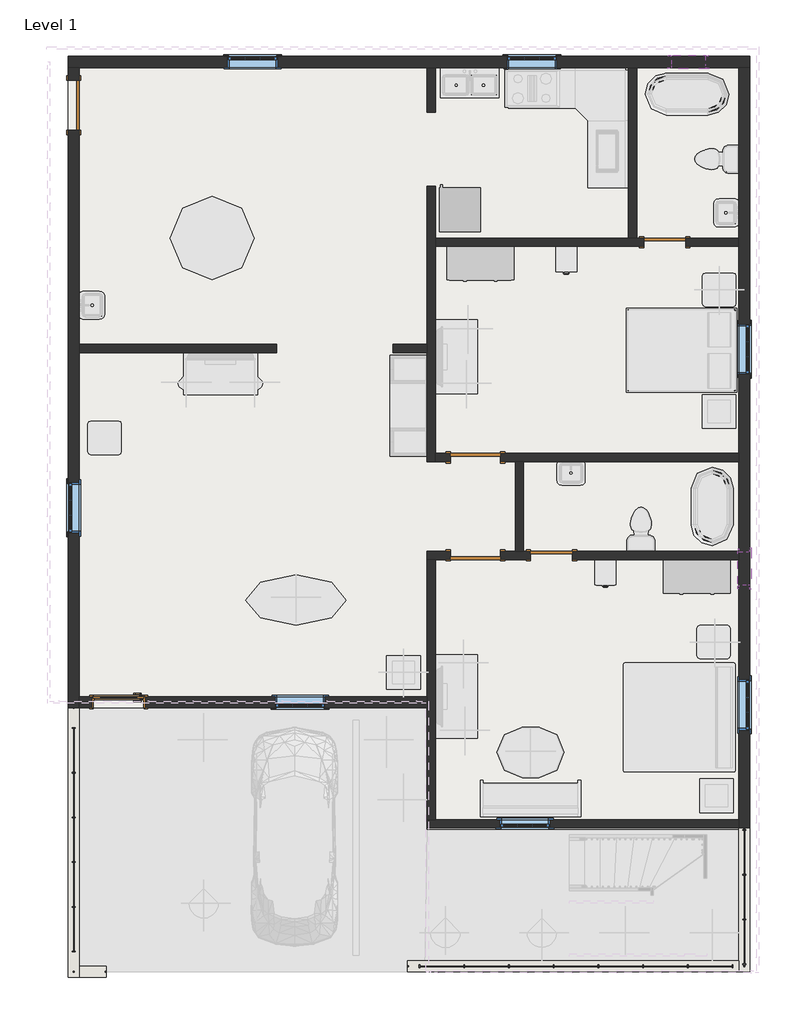
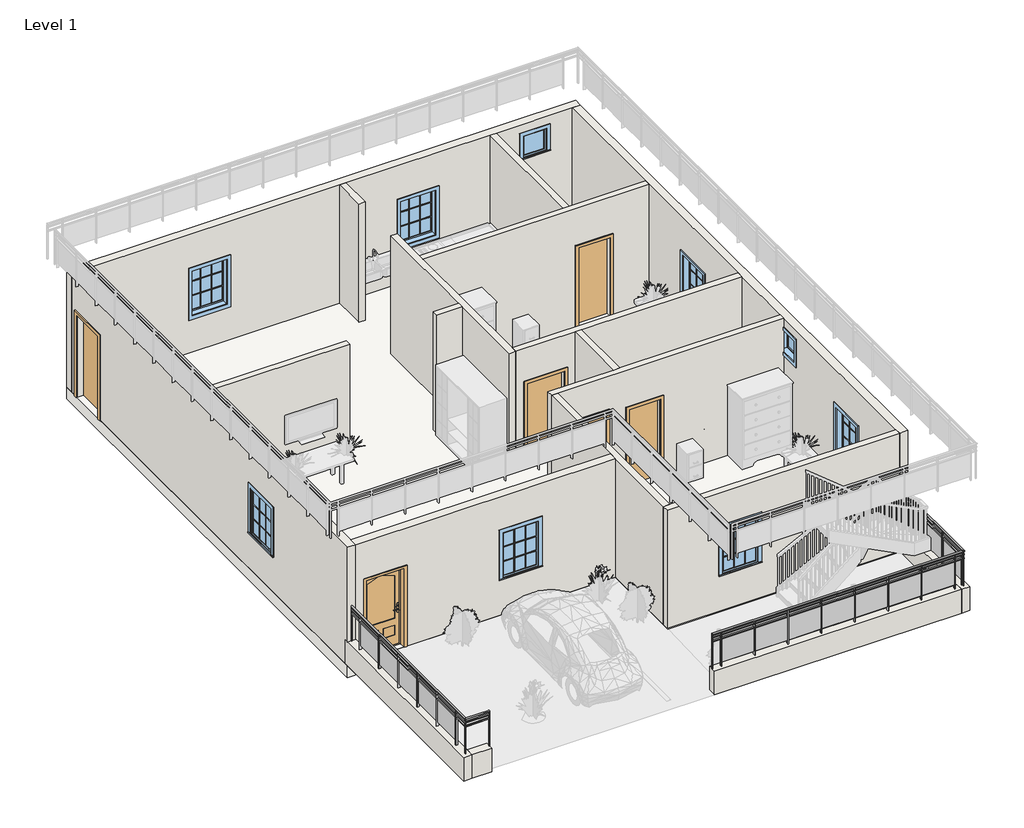
# One storey, part 1 of 5: 19 walls, 9 windows, 6 doors, 2 railings, 1 slab.
# Revit data of these elements (continued)
# Element 31 (IfcWindow, "Casement 3x3 with Trim : 36\" x 48\"")
#   Mark = "3"
#   Phase Created = New Construction
#   Materials on its faces: "Sash", "Glass", "Trim"
# Element 32 (IfcWindow, "Casement 3x3 with Trim : 36\" x 48\"")
#   Mark = "4"
#   Phase Created = New Construction
#   Materials on its faces: "Sash", "Glass", "Trim"
# Element 33 (IfcWindow, "Casement 3x3 with Trim : 36\" x 48\"")
#   Mark = "5"
#   Phase Created = New Construction
#   Materials on its faces: "Sash", "Glass", "Trim"
# Element 34 (IfcWindow, "Casement 3x3 with Trim : 36\" x 48\"")
#   Mark = "6"
#   Phase Created = New Construction
#   Materials on its faces: "Sash", "Glass", "Trim"
# Element 35 (IfcWindow, "Casement 3x3 with Trim : 36\" x 48\"")
#   Mark = "9"
#   Phase Created = New Construction
#   Materials on its faces: "Sash", "Glass", "Trim"
# Element 36 (IfcWindow, "Transom with Trim : 24\" x 24\"")
#   Mark = "7"
#   Phase Created = New Construction
#   Materials on its faces: "Sash", "Trim", "Glass"
# Element 37 (IfcWindow, "Transom with Trim : 24\" x 24\"")
#   Mark = "8"
#   Phase Created = New Construction
#   Materials on its faces: "Sash", "Trim", "Glass"
# Materials
#   "Cherry": class "Wood", colour RGB 226 177 128, transparency 0, Description = "Prunus Serotina", Cost = 0
#   "Glass": class "Glass", colour RGB 0 128 192, transparency 0.75, Description = "Soda Lime Glass", Cost = 0
#   "Aluminum": class "Metal", colour RGB 247 247 247, transparency 0, Description = "Aluminum 6061", Cost = 0
#   "Door - Panel": class "Wood", colour RGB 210 159 95, transparency 0
#   "Door - Frame": colour RGB 118 70 51, transparency 0
#   "Birch": class "Wood", colour RGB 210 159 95, transparency 0, Description = "Betula Alleghaniensis", Cost = 0
#   "Brick, Common": class "Masonry", colour RGB 170 98 104, transparency 0, Description = "Common brick", Cost = 0
#   "Sash": class "Wood", colour RGB 224 178 126, transparency 0
#   "Trim": class "Wood", colour RGB 224 178 126, transparency 0
#   "Default Floor": colour RGB 128 128 128, transparency 0
# Room at (-3943.75, 11818.36) mm, phase "New Construction", upper level "Level 1", upper offset 10' - 0", lower offset 0' - 0"
#   Number = "2"
#   Name = "OPEN KITCHEN"
# Room at (-1063.794, 12123.16) mm, phase "New Construction", upper level "Level 1", upper offset 10' - 0", lower offset 0' - 0"
#   Number = "3"
# Room at (-3126.869, 8673.263) mm, phase "New Construction", upper level "Level 1", upper offset 10' - 0", lower offset 0' - 0"
#   Number = "4"
# Room at (-2226.29, 5725.647) mm, phase "New Construction", upper level "Level 1", upper offset 10' - 0", lower offset 0' - 0"
#   Number = "5"
# Room at (-2944.225, 2474.386) mm, phase "New Construction", upper level "Level 1", upper offset 10' - 0", lower offset 0' - 0"
#   Number = "6"
# Room at (-8666.158, 5725.647) mm, phase "New Construction", upper level "Level 1", upper offset 10' - 0", lower offset 0' - 0"
#   Number = "7"
#   Name = "LIVING HALL"
# Room at (-8922.617, 11470.605) mm, phase "New Construction", upper level "Level 1", upper offset 10' - 0", lower offset 0' - 0"
#   Number = "1"
#   Name = "DINING HALL"
